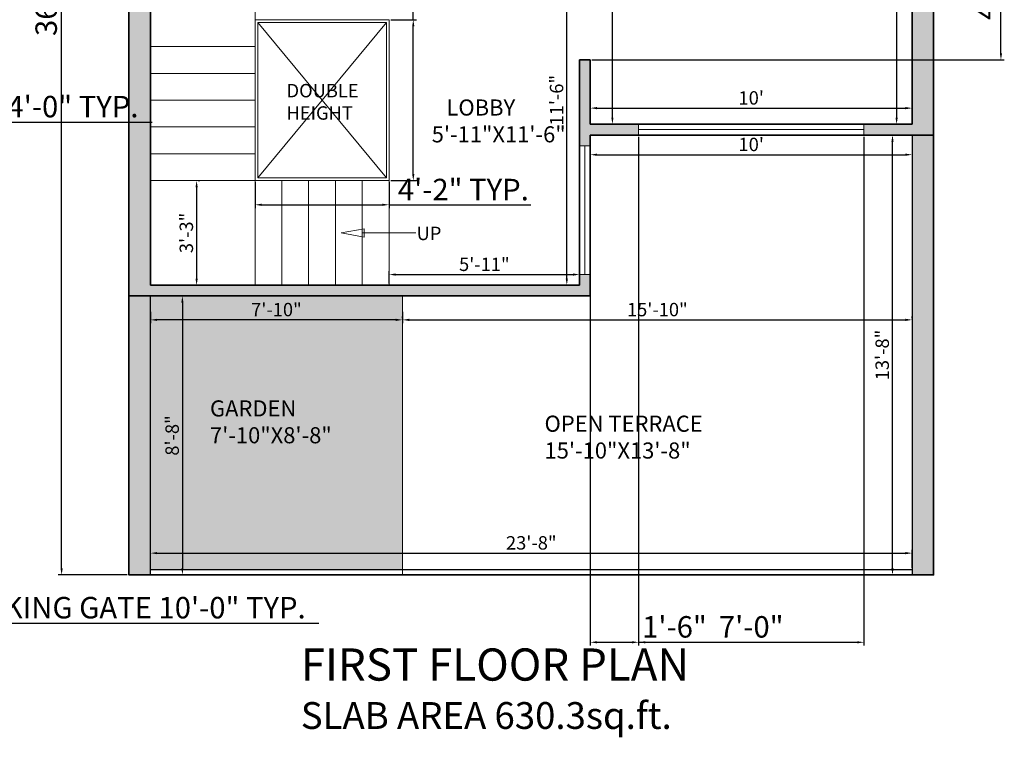
# Model space of a CAD drawing. Units: inches. Extents: x 3259 to 4981, y 1402 to 2026.
# Tile 10 of 11: x 4614 to 4981, y 1415 to 1682. Entities that reach past the tile are written whole.
import ezdxf

# ---------------------------------------------------------------- set-up
doc = ezdxf.new("R2010")
doc.units = ezdxf.units.IN
for name, color, linetype, lineweight in [('A-ANNO-DIMS', 2, 'Continuous', 13), ('A-ANNO-SYMB', 7, 'Continuous', 13), ('A-ANNO-TITL', 7, 'Continuous', 25), ('A-AREA-IDEN', 7, 'Continuous', 18), ('A-DOOR', 3, 'Continuous', 18), ('A-FLOR-STRS', 7, 'Continuous', 18), ('A-GLAZ', 4, 'Continuous', 18), ('A-WALL', 7, 'Continuous', 35), ('A-WALL-PATT', 252, 'Continuous', 13), ('A-WALL-PRPT', 7, 'Continuous', 25), ('L-PLNT', 3, 'Continuous', 18)]:
    doc.layers.add(name, color=color, linetype=linetype, lineweight=lineweight)
doc.layers.add('A-WALL-PRPT-PATT', color=9, linetype='Continuous', lineweight=13, true_color=0xc7c8ca)
doc.layers.add('L-PLNT-PATT', color=114, linetype='Continuous', lineweight=13, true_color=0x139b48)
doc.styles.get("Standard").update_dxf_attribs({"font": 'arial.ttf'})
doc.dimstyles.new('ISO-25', dxfattribs={"dimtxt": 8, "dimasz": 2.5, "dimexe": 1.25, "dimexo": 0.625, "dimtad": 1, "dimdec": 1, "dimlunit": 3, "dimtxsty": 'Standard', "dimcen": 2.5, "dimclrd": 4, "dimclre": 4, "dimclrt": 1, "dimadec": 0, "dimazin": 0, "dimtfac": 1, "dimtdec": 1, "dimtmove": 0, "dimatfit": 3, "dimfxl": 1, "dimarcsym": 0})

# ---------------------------------------------------------------- blocks, each defined once
blk = doc.blocks.new('*D90')
at = {"layer": 'A-ANNO-DIMS', "color": 0, "lineweight": -2, "transparency": 16777216}
for p, q in [((4662.83, 1573.27), (4662.83, 1568.97)), ((4756.83, 1573.27), (4756.83, 1568.97)), ((4754.33, 1570.22), (4665.33, 1570.22))]:
    blk.add_line(p, q, dxfattribs=at)
at = {"layer": 'A-ANNO-DIMS', "color": 0, "transparency": 16777216}
for points in [[(4665.33, 1570.63), (4665.33, 1569.8), (4662.83, 1570.22)], [(4754.33, 1570.63), (4754.33, 1569.8), (4756.83, 1570.22)]]:
    blk.add_solid(points, dxfattribs=at)
at = {"layer": 'Defpoints', "color": 0, "transparency": 16777216}
for p in [(4662.83, 1573.89), (4756.83, 1573.89), (4662.83, 1570.22)]:
    blk.add_point(p, dxfattribs=at)
at = {"layer": 'A-ANNO-DIMS', "color": 0, "transparency": 16777216, "insert": (4709.83, 1573.4), "char_height": 5, "attachment_point": 5}
blk.add_mtext('7\'-10"', dxfattribs=at)
blk = doc.blocks.new('*D91')
at = {"layer": 'A-ANNO-DIMS', "color": 0, "lineweight": -2, "transparency": 16777216}
for p, q in [((4673.41, 1579.12), (4676.02, 1579.12)), ((4674.77, 1576.62), (4674.77, 1477.62)), ((4673.41, 1475.12), (4676.02, 1475.12))]:
    blk.add_line(p, q, dxfattribs=at)
at = {"layer": 'A-ANNO-DIMS', "color": 0, "transparency": 16777216}
for points in [[(4674.35, 1576.62), (4675.18, 1576.62), (4674.77, 1579.12)], [(4674.35, 1477.62), (4675.18, 1477.62), (4674.77, 1475.12)]]:
    blk.add_solid(points, dxfattribs=at)
at = {"layer": 'Defpoints', "color": 0, "transparency": 16777216}
for p in [(4672.79, 1579.12), (4672.79, 1475.12), (4674.77, 1475.12)]:
    blk.add_point(p, dxfattribs=at)
at = {"layer": 'A-ANNO-DIMS', "color": 0, "transparency": 16777216, "insert": (4671.59, 1527.12), "char_height": 5, "attachment_point": 5, "rotation": 90}
blk.add_mtext('8\'-8"', dxfattribs=at)
blk = doc.blocks.new('*D92')
at = {"layer": 'A-ANNO-DIMS', "color": 0, "lineweight": -2, "transparency": 16777216}
for p, q in [((4756.83, 1570.84), (4756.83, 1571.47)), ((4946.83, 1570.84), (4946.83, 1571.47)), ((4759.33, 1570.22), (4944.33, 1570.22))]:
    blk.add_line(p, q, dxfattribs=at)
at = {"layer": 'A-ANNO-DIMS', "color": 0, "transparency": 16777216}
for points in [[(4759.33, 1570.63), (4759.33, 1569.8), (4756.83, 1570.22)], [(4944.33, 1570.63), (4944.33, 1569.8), (4946.83, 1570.22)]]:
    blk.add_solid(points, dxfattribs=at)
at = {"layer": 'Defpoints', "color": 0, "transparency": 16777216}
for p in [(4756.83, 1570.22), (4946.83, 1570.22), (4946.83, 1570.22)]:
    blk.add_point(p, dxfattribs=at)
at = {"layer": 'A-ANNO-DIMS', "color": 0, "transparency": 16777216, "insert": (4851.83, 1573.4), "char_height": 5, "attachment_point": 5}
blk.add_mtext('15\'-10"', dxfattribs=at)
blk = doc.blocks.new('*D93')
at = {"layer": 'A-ANNO-DIMS', "color": 0, "lineweight": -2, "transparency": 16777216}
for p, q in [((4946.2, 1639.12), (4938.24, 1639.12)), ((4939.49, 1477.62), (4939.49, 1636.62)), ((4946.2, 1475.12), (4938.24, 1475.12))]:
    blk.add_line(p, q, dxfattribs=at)
at = {"layer": 'A-ANNO-DIMS', "color": 0, "transparency": 16777216}
for points in [[(4939.08, 1636.62), (4939.91, 1636.62), (4939.49, 1639.12)], [(4939.08, 1477.62), (4939.91, 1477.62), (4939.49, 1475.12)]]:
    blk.add_solid(points, dxfattribs=at)
at = {"layer": 'Defpoints', "color": 0, "transparency": 16777216}
for p in [(4939.49, 1639.12), (4946.83, 1639.12), (4946.83, 1475.12)]:
    blk.add_point(p, dxfattribs=at)
at = {"layer": 'A-ANNO-DIMS', "color": 0, "transparency": 16777216, "insert": (4936.31, 1557.12), "char_height": 5, "attachment_point": 5, "rotation": 90}
blk.add_mtext('13\'-8"', dxfattribs=at)
blk = doc.blocks.new('*D85')
at = {"layer": 'A-ANNO-DIMS', "color": 0, "lineweight": -2, "transparency": 16777216}
for p, q in [((4751.83, 1583.74), (4751.83, 1588.35)), ((4754.33, 1587.1), (4820.33, 1587.1)), ((4822.83, 1583.74), (4822.83, 1588.35))]:
    blk.add_line(p, q, dxfattribs=at)
at = {"layer": 'A-ANNO-DIMS', "color": 0, "transparency": 16777216}
for points in [[(4754.33, 1587.52), (4754.33, 1586.68), (4751.83, 1587.1)], [(4820.33, 1587.52), (4820.33, 1586.68), (4822.83, 1587.1)]]:
    blk.add_solid(points, dxfattribs=at)
at = {"layer": 'Defpoints', "color": 0, "transparency": 16777216}
for p in [(4822.83, 1587.1), (4751.83, 1583.12), (4822.83, 1583.12)]:
    blk.add_point(p, dxfattribs=at)
at = {"layer": 'A-ANNO-DIMS', "color": 0, "transparency": 16777216, "insert": (4787.33, 1590.28), "char_height": 5, "attachment_point": 5}
blk.add_mtext('5\'-11"', dxfattribs=at)
blk = doc.blocks.new('*D86')
at = {"layer": 'A-ANNO-DIMS', "color": 0, "lineweight": -2, "transparency": 16777216}
for p, q in [((4787.45, 1721.12), (4819.32, 1721.12)), ((4818.07, 1585.62), (4818.07, 1718.62)), ((4822.2, 1583.12), (4816.82, 1583.12))]:
    blk.add_line(p, q, dxfattribs=at)
at = {"layer": 'A-ANNO-DIMS', "color": 0, "transparency": 16777216}
for points in [[(4817.66, 1718.62), (4818.49, 1718.62), (4818.07, 1721.12)], [(4817.66, 1585.62), (4818.49, 1585.62), (4818.07, 1583.12)]]:
    blk.add_solid(points, dxfattribs=at)
at = {"layer": 'Defpoints', "color": 0, "transparency": 16777216}
for p in [(4786.83, 1721.12), (4818.07, 1721.12), (4822.83, 1583.12)]:
    blk.add_point(p, dxfattribs=at)
at = {"layer": 'A-ANNO-DIMS', "color": 0, "transparency": 16777216, "insert": (4814.9, 1652.12), "char_height": 5, "attachment_point": 5, "rotation": 90}
blk.add_mtext('11\'-6"', dxfattribs=at)
blk = doc.blocks.new('*D87')
at = {"layer": 'A-ANNO-DIMS', "color": 0, "lineweight": -2, "transparency": 16777216}
for p, q in [((4826.83, 1643.74), (4826.83, 1650.4)), ((4829.33, 1649.15), (4944.33, 1649.15)), ((4946.83, 1643.74), (4946.83, 1650.4))]:
    blk.add_line(p, q, dxfattribs=at)
at = {"layer": 'A-ANNO-DIMS', "color": 0, "transparency": 16777216}
for points in [[(4829.33, 1649.56), (4829.33, 1648.73), (4826.83, 1649.15)], [(4944.33, 1649.56), (4944.33, 1648.73), (4946.83, 1649.15)]]:
    blk.add_solid(points, dxfattribs=at)
at = {"layer": 'Defpoints', "color": 0, "transparency": 16777216}
for p in [(4946.83, 1649.15), (4826.83, 1643.12), (4946.83, 1643.12)]:
    blk.add_point(p, dxfattribs=at)
at = {"layer": 'A-ANNO-DIMS', "color": 0, "transparency": 16777216, "insert": (4886.83, 1652.32), "char_height": 5, "attachment_point": 5}
blk.add_mtext("10'", dxfattribs=at)
blk = doc.blocks.new('*D88')
at = {"layer": 'A-ANNO-DIMS', "color": 0, "lineweight": -2, "transparency": 16777216}
for p, q in [((4827.45, 1847.12), (4836.33, 1847.12)), ((4835.08, 1645.62), (4835.08, 1844.62)), ((4827.45, 1643.12), (4836.33, 1643.12))]:
    blk.add_line(p, q, dxfattribs=at)
at = {"layer": 'A-ANNO-DIMS', "color": 0, "transparency": 16777216}
for points in [[(4834.66, 1844.62), (4835.49, 1844.62), (4835.08, 1847.12)], [(4834.66, 1645.62), (4835.49, 1645.62), (4835.08, 1643.12)]]:
    blk.add_solid(points, dxfattribs=at)
at = {"layer": 'Defpoints', "color": 0, "transparency": 16777216}
for p in [(4826.83, 1847.12), (4835.08, 1847.12), (4826.83, 1643.12)]:
    blk.add_point(p, dxfattribs=at)
at = {"layer": 'A-ANNO-DIMS', "color": 0, "transparency": 16777216, "insert": (4831.94, 1745.12), "char_height": 5, "attachment_point": 5, "rotation": 90}
blk.add_mtext("17'", dxfattribs=at)
blk = doc.blocks.new('*D94')
at = {"layer": 'A-ANNO-DIMS', "color": 0, "lineweight": -2, "transparency": 16777216}
for p, q in [((4680.06, 1619.62), (4680.06, 1585.62)), ((4680.69, 1622.12), (4681.31, 1622.12)), ((4680.69, 1583.12), (4681.31, 1583.12))]:
    blk.add_line(p, q, dxfattribs=at)
at = {"layer": 'A-ANNO-DIMS', "color": 0, "transparency": 16777216}
for points in [[(4679.64, 1619.62), (4680.48, 1619.62), (4680.06, 1622.12)], [(4679.64, 1585.62), (4680.48, 1585.62), (4680.06, 1583.12)]]:
    blk.add_solid(points, dxfattribs=at)
at = {"layer": 'Defpoints', "color": 0, "transparency": 16777216}
for p in [(4680.06, 1622.12), (4680.06, 1583.12), (4680.06, 1583.12)]:
    blk.add_point(p, dxfattribs=at)
at = {"layer": 'A-ANNO-DIMS', "color": 0, "transparency": 16777216, "insert": (4676.88, 1602.62), "char_height": 5, "attachment_point": 5, "rotation": 90}
blk.add_mtext('3\'-3"', dxfattribs=at)
blk = doc.blocks.new('*D63')
at = {"layer": 'A-ANNO-DIMS', "color": 0, "lineweight": -2, "transparency": 16777216}
for p, q in [((4826.83, 1638.49), (4826.83, 1630.53)), ((4946.83, 1638.49), (4946.83, 1630.53)), ((4829.33, 1631.78), (4944.33, 1631.78))]:
    blk.add_line(p, q, dxfattribs=at)
at = {"layer": 'A-ANNO-DIMS', "color": 0, "transparency": 16777216}
for points in [[(4829.33, 1632.2), (4829.33, 1631.37), (4826.83, 1631.78)], [(4944.33, 1632.2), (4944.33, 1631.37), (4946.83, 1631.78)]]:
    blk.add_solid(points, dxfattribs=at)
at = {"layer": 'Defpoints', "color": 0, "transparency": 16777216}
for p in [(4826.83, 1639.12), (4946.83, 1639.12), (4946.83, 1631.78)]:
    blk.add_point(p, dxfattribs=at)
at = {"layer": 'A-ANNO-DIMS', "color": 0, "transparency": 16777216, "insert": (4886.83, 1634.96), "char_height": 5, "attachment_point": 5}
blk.add_mtext("10'", dxfattribs=at)
blk = doc.blocks.new('*D99')
at = {"layer": 'A-ANNO-DIMS', "color": 0, "lineweight": -2, "transparency": 16777216}
for p, q in [((4946.2, 1847.12), (4939.77, 1847.12)), ((4941.02, 1844.62), (4941.02, 1645.62)), ((4946.2, 1643.12), (4939.77, 1643.12))]:
    blk.add_line(p, q, dxfattribs=at)
at = {"layer": 'A-ANNO-DIMS', "color": 0, "transparency": 16777216}
for points in [[(4940.61, 1844.62), (4941.44, 1844.62), (4941.02, 1847.12)], [(4940.61, 1645.62), (4941.44, 1645.62), (4941.02, 1643.12)]]:
    blk.add_solid(points, dxfattribs=at)
at = {"layer": 'Defpoints', "color": 0, "transparency": 16777216}
for p in [(4946.83, 1847.12), (4941.02, 1643.12), (4946.83, 1643.12)]:
    blk.add_point(p, dxfattribs=at)
at = {"layer": 'A-ANNO-DIMS', "color": 0, "transparency": 16777216, "insert": (4937.89, 1745.12), "char_height": 5, "attachment_point": 5, "rotation": 90}
blk.add_mtext("17'", dxfattribs=at)
blk = doc.blocks.new('*D133')
at = {"layer": 'A-ANNO-DIMS', "color": 0, "lineweight": -2, "transparency": 16777216}
for p, q in [((4662.83, 1477.74), (4662.83, 1484.5)), ((4665.33, 1483.25), (4944.33, 1483.25)), ((4946.83, 1477.74), (4946.83, 1484.5))]:
    blk.add_line(p, q, dxfattribs=at)
at = {"layer": 'A-ANNO-DIMS', "color": 0, "transparency": 16777216}
for points in [[(4665.33, 1483.67), (4665.33, 1482.84), (4662.83, 1483.25)], [(4944.33, 1483.67), (4944.33, 1482.84), (4946.83, 1483.25)]]:
    blk.add_solid(points, dxfattribs=at)
at = {"layer": 'Defpoints', "color": 0, "transparency": 16777216}
for p in [(4946.83, 1483.25), (4662.83, 1477.12), (4946.83, 1477.12)]:
    blk.add_point(p, dxfattribs=at)
at = {"layer": 'A-ANNO-DIMS', "color": 0, "transparency": 16777216, "insert": (4804.83, 1486.43), "char_height": 5, "attachment_point": 5}
blk.add_mtext('23\'-8"', dxfattribs=at)
blk = doc.blocks.new('STAIR-WELL-50x60')
for p, q in [((1, 59), (49, 1)), ((1, 1), (49, 59))]:
    blk.add_line(p, q)
for points in [[(50, 60), (0, 60), (0, 0), (50, 0)], [(49, 59), (1, 59), (1, 1), (49, 1)]]:
    blk.add_lwpolyline(points, close=True)
blk = doc.blocks.new('STAIR-DIRECTION')
blk.add_line((7.93, 1.55), (27.85, 1.55))
blk.add_lwpolyline([(0, 1.55), (8.64, 3.11), (8.64, 0)], close=True)
blk = doc.blocks.new('*D154')
at = {"layer": 'A-ANNO-DIMS', "color": 4, "lineweight": -2, "transparency": 16777216}
for p, q in [((4760.83, 1682.12), (4760.83, 1804.15)), ((4752.45, 1682.12), (4762.08, 1682.12)), ((4760.83, 1624.62), (4760.83, 1679.62)), ((4752.45, 1622.12), (4762.08, 1622.12))]:
    blk.add_line(p, q, dxfattribs=at)
at = {"layer": 'A-ANNO-DIMS', "color": 4, "transparency": 16777216}
for points in [[(4760.41, 1679.62), (4761.25, 1679.62), (4760.83, 1682.12)], [(4760.41, 1624.62), (4761.25, 1624.62), (4760.83, 1622.12)]]:
    blk.add_solid(points, dxfattribs=at)
at = {"layer": 'Defpoints', "color": 0, "transparency": 16777216}
for p in [(4751.83, 1682.12), (4760.83, 1682.12), (4751.83, 1622.12)]:
    blk.add_point(p, dxfattribs=at)
at = {"layer": 'A-ANNO-DIMS', "color": 1, "transparency": 16777216, "insert": (4756.07, 1744.38), "char_height": 8, "attachment_point": 5, "rotation": 90}
blk.add_mtext('STAIR WELL 5\'-0" TYP.', dxfattribs=at)
blk = doc.blocks.new('*D155')
at = {"layer": 'A-ANNO-DIMS', "color": 4, "lineweight": -2, "transparency": 16777216}
for p, q in [((4701.83, 1621.49), (4701.83, 1611.87)), ((4751.83, 1621.49), (4751.83, 1611.87)), ((4704.33, 1613.12), (4749.33, 1613.12)), ((4751.83, 1613.12), (4804.67, 1613.12))]:
    blk.add_line(p, q, dxfattribs=at)
at = {"layer": 'A-ANNO-DIMS', "color": 4, "transparency": 16777216}
for points in [[(4704.33, 1613.53), (4704.33, 1612.7), (4701.83, 1613.12)], [(4749.33, 1613.53), (4749.33, 1612.7), (4751.83, 1613.12)]]:
    blk.add_solid(points, dxfattribs=at)
at = {"layer": 'Defpoints', "color": 0, "transparency": 16777216}
for p in [(4701.83, 1622.12), (4751.83, 1622.12), (4751.83, 1613.12)]:
    blk.add_point(p, dxfattribs=at)
at = {"layer": 'A-ANNO-DIMS', "color": 1, "transparency": 16777216, "insert": (4779.5, 1617.76), "char_height": 8, "attachment_point": 5}
blk.add_mtext('4\'-2" TYP.', dxfattribs=at)
blk = doc.blocks.new('*D170')
at = {"layer": 'A-ANNO-DIMS', "color": 4, "lineweight": -2, "transparency": 16777216}
for p, q in [((4478.33, 1650.49), (4478.33, 1642.67)), ((4526.33, 1650.49), (4526.33, 1642.67)), ((4480.83, 1643.92), (4523.83, 1643.92)), ((4526.33, 1643.92), (4663.49, 1643.92))]:
    blk.add_line(p, q, dxfattribs=at)
at = {"layer": 'A-ANNO-DIMS', "color": 4, "transparency": 16777216}
for points in [[(4480.83, 1644.33), (4480.83, 1643.5), (4478.33, 1643.92)], [(4523.83, 1644.33), (4523.83, 1643.5), (4526.33, 1643.92)]]:
    blk.add_solid(points, dxfattribs=at)
at = {"layer": 'Defpoints', "color": 0, "transparency": 16777216}
for p in [(4478.33, 1651.12), (4526.33, 1651.12), (4526.33, 1643.92)]:
    blk.add_point(p, dxfattribs=at)
at = {"layer": 'A-ANNO-DIMS', "color": 1, "transparency": 16777216, "insert": (4596.16, 1648.68), "char_height": 8, "attachment_point": 5}
blk.add_mtext('ENTRY DOORS 4\'-0" TYP.', dxfattribs=at)
blk = doc.blocks.new('*D172')
at = {"layer": 'A-ANNO-DIMS', "color": 4, "lineweight": -2, "transparency": 16777216}
for p, q in [((4460.33, 1474.49), (4460.33, 1455.87)), ((4580.33, 1474.49), (4580.33, 1455.87)), ((4462.83, 1457.12), (4577.83, 1457.12)), ((4580.33, 1457.12), (4725.6, 1457.12))]:
    blk.add_line(p, q, dxfattribs=at)
at = {"layer": 'A-ANNO-DIMS', "color": 4, "transparency": 16777216}
for points in [[(4462.83, 1457.53), (4462.83, 1456.7), (4460.33, 1457.12)], [(4577.83, 1457.53), (4577.83, 1456.7), (4580.33, 1457.12)]]:
    blk.add_solid(points, dxfattribs=at)
at = {"layer": 'Defpoints', "color": 0, "transparency": 16777216}
for p in [(4460.33, 1475.12), (4580.33, 1475.12), (4580.33, 1457.12)]:
    blk.add_point(p, dxfattribs=at)
at = {"layer": 'A-ANNO-DIMS', "color": 1, "transparency": 16777216, "insert": (4654.22, 1461.88), "char_height": 8, "attachment_point": 5}
blk.add_mtext('PARKING GATE 10\'-0" TYP.', dxfattribs=at)
blk = doc.blocks.new('*D189')
at = {"layer": 'A-ANNO-DIMS', "color": 4, "lineweight": -2, "transparency": 16777216}
for p, q in [((4654.2, 1907.12), (4628.48, 1907.12)), ((4629.73, 1477.62), (4629.73, 1904.62)), ((4654.2, 1475.12), (4628.48, 1475.12))]:
    blk.add_line(p, q, dxfattribs=at)
at = {"layer": 'A-ANNO-DIMS', "color": 4, "transparency": 16777216}
for points in [[(4629.31, 1904.62), (4630.15, 1904.62), (4629.73, 1907.12)], [(4629.31, 1477.62), (4630.15, 1477.62), (4629.73, 1475.12)]]:
    blk.add_solid(points, dxfattribs=at)
at = {"layer": 'Defpoints', "color": 0, "transparency": 16777216}
for p in [(4629.73, 1907.12), (4654.83, 1907.12), (4654.83, 1475.12)]:
    blk.add_point(p, dxfattribs=at)
at = {"layer": 'A-ANNO-DIMS', "color": 1, "transparency": 16777216, "insert": (4625.02, 1691.12), "char_height": 8, "attachment_point": 5, "rotation": 90}
blk.add_mtext('36\'-0"', dxfattribs=at)
blk = doc.blocks.new('*D197')
at = {"layer": 'A-ANNO-DIMS', "color": 4, "lineweight": -2, "transparency": 16777216}
for p, q in [((4827.45, 1721.12), (4981.18, 1721.12)), ((4979.93, 1669.62), (4979.93, 1718.62)), ((4827.45, 1667.12), (4981.18, 1667.12))]:
    blk.add_line(p, q, dxfattribs=at)
at = {"layer": 'A-ANNO-DIMS', "color": 4, "transparency": 16777216}
for points in [[(4979.51, 1718.62), (4980.35, 1718.62), (4979.93, 1721.12)], [(4979.51, 1669.62), (4980.35, 1669.62), (4979.93, 1667.12)]]:
    blk.add_solid(points, dxfattribs=at)
at = {"layer": 'Defpoints', "color": 0, "transparency": 16777216}
for p in [(4826.83, 1721.12), (4979.93, 1721.12), (4826.83, 1667.12)]:
    blk.add_point(p, dxfattribs=at)
at = {"layer": 'A-ANNO-DIMS', "color": 1, "transparency": 16777216, "insert": (4975.22, 1694.12), "char_height": 8, "attachment_point": 5, "rotation": 90}
blk.add_mtext('4\'-6"', dxfattribs=at)
blk = doc.blocks.new('*D198')
at = {"layer": 'A-ANNO-DIMS', "color": 4, "lineweight": -2, "transparency": 16777216}
for p, q in [((4844.83, 1638.49), (4844.83, 1448.77)), ((4928.83, 1638.49), (4928.83, 1448.77)), ((4847.33, 1450.02), (4926.33, 1450.02))]:
    blk.add_line(p, q, dxfattribs=at)
at = {"layer": 'A-ANNO-DIMS', "color": 4, "transparency": 16777216}
for points in [[(4847.33, 1450.43), (4847.33, 1449.6), (4844.83, 1450.02)], [(4926.33, 1450.43), (4926.33, 1449.6), (4928.83, 1450.02)]]:
    blk.add_solid(points, dxfattribs=at)
at = {"layer": 'Defpoints', "color": 0, "transparency": 16777216}
for p in [(4844.83, 1639.12), (4928.83, 1639.12), (4928.83, 1450.02)]:
    blk.add_point(p, dxfattribs=at)
at = {"layer": 'A-ANNO-DIMS', "color": 1, "transparency": 16777216, "insert": (4886.83, 1454.73), "char_height": 8, "attachment_point": 5}
blk.add_mtext('7\'-0"', dxfattribs=at)
blk = doc.blocks.new('*D199')
at = {"layer": 'A-ANNO-DIMS', "color": 4, "lineweight": -2, "transparency": 16777216}
for p, q in [((4826.83, 1638.49), (4826.83, 1448.77)), ((4844.83, 1638.49), (4844.83, 1448.77)), ((4829.33, 1450.02), (4842.33, 1450.02)), ((4844.83, 1450.02), (4869.09, 1450.02))]:
    blk.add_line(p, q, dxfattribs=at)
at = {"layer": 'A-ANNO-DIMS', "color": 4, "transparency": 16777216}
for points in [[(4829.33, 1450.43), (4829.33, 1449.6), (4826.83, 1450.02)], [(4842.33, 1450.43), (4842.33, 1449.6), (4844.83, 1450.02)]]:
    blk.add_solid(points, dxfattribs=at)
at = {"layer": 'Defpoints', "color": 0, "transparency": 16777216}
for p in [(4826.83, 1639.12), (4844.83, 1639.12), (4844.83, 1450.02)]:
    blk.add_point(p, dxfattribs=at)
at = {"layer": 'A-ANNO-DIMS', "color": 1, "transparency": 16777216, "insert": (4858.21, 1454.73), "char_height": 8, "attachment_point": 5}
blk.add_mtext('1\'-6"', dxfattribs=at)

msp = doc.modelspace()

# ---------------------------------------------------------------- hatches: boundary and pattern name
at = {"layer": 'A-WALL-PATT'}
h = msp.add_hatch(color=256, dxfattribs=at)
h.dxf.hatch_style = 1
h.paths.add_polyline_path([(4826.83, 1851.12), (4822.83, 1851.12), (4822.83, 1721.12), (4826.83, 1721.12), (4826.83, 1777.43), (4826.82, 1777.43), (4826.82, 1777.47), (4826.83, 1777.47), (4826.83, 1781.5), (4826.83, 1781.5), (4826.83, 1781.55)], flags=17)
h.paths.add_polyline_path([(4786.83, 1863.12), (4782.83, 1863.12), (4782.83, 1851.12), (4698.83, 1851.12), (4698.83, 1847.12), (4736.66, 1847.12), (4736.66, 1847.13), (4736.7, 1847.13), (4736.7, 1847.12), (4740.73, 1847.12), (4740.73, 1847.12), (4740.78, 1847.12), (4786.83, 1847.12)], flags=17)
h.paths.add_polyline_path([(4862.83, 1863.12), (4858.83, 1863.12), (4858.83, 1847.12), (4862.83, 1847.12)], flags=17)
h.paths.add_polyline_path([(4954.83, 1907.12), (4654.83, 1907.12), (4654.83, 1579.12), (4826.83, 1579.12), (4826.83, 1587.12), (4822.83, 1587.12), (4822.83, 1583.12), (4662.83, 1583.12), (4662.83, 1721.12), (4786.83, 1721.12), (4786.83, 1725.12), (4662.83, 1725.12), (4662.83, 1899.12), (4698.83, 1899.12), (4698.83, 1881.12), (4702.83, 1881.12), (4702.83, 1899.12), (4782.83, 1899.12), (4782.83, 1887.12), (4786.83, 1887.12), (4786.83, 1899.12), (4858.83, 1899.12), (4858.83, 1887.12), (4862.83, 1887.12), (4862.83, 1899.12), (4946.83, 1899.12), (4946.83, 1851.12), (4892.83, 1851.12), (4892.83, 1847.12), (4946.83, 1847.12), (4946.83, 1643.12), (4928.83, 1643.12), (4928.83, 1639.12), (4954.83, 1639.12)])
h.paths.add_polyline_path([(4826.83, 1667.12), (4822.83, 1667.12), (4822.83, 1635.12), (4826.83, 1635.12), (4826.83, 1639.12), (4844.83, 1639.12), (4844.83, 1643.12), (4826.83, 1643.12)], flags=17)
at = {"layer": 'A-WALL-PRPT-PATT'}
h = msp.add_hatch(color=256, dxfattribs=at)
h.dxf.hatch_style = 1
h.paths.add_polyline_path([(4954.83, 1639.12), (4946.83, 1639.12), (4946.83, 1475.12), (4954.83, 1475.12)])
h.paths.add_polyline_path([(4662.83, 1579.12), (4654.83, 1579.12), (4654.83, 1475.12), (4662.83, 1475.12)])
at = {"layer": 'L-PLNT-PATT'}
h = msp.add_hatch(color=256, dxfattribs=at)
h.dxf.hatch_style = 1
h.paths.add_polyline_path([(4756.83, 1579.12), (4662.83, 1579.12), (4662.83, 1477.12), (4756.83, 1477.12)])
h.paths.add_polyline_path([(4683.1, 1520.8), (4729.79, 1520.8), (4729.79, 1543.19), (4683.1, 1543.19)], flags=24)

# ---------------------------------------------------------------- linework, layer by layer
at = {"layer": 'A-DOOR'}
for p, q in [((4822.83, 1635.12), (4826.83, 1635.12)), ((4824.83, 1635.12), (4824.83, 1587.12)), ((4826.83, 1587.12), (4822.83, 1587.12))]:
    msp.add_line(p, q, dxfattribs=at)
at = {"layer": 'A-FLOR-STRS'}
for p, q in [((4701.83, 1583.12), (4701.83, 1721.12)), ((4662.83, 1672.12), (4701.83, 1672.12)), ((4662.83, 1662.12), (4701.83, 1662.12)), ((4662.83, 1652.12), (4701.83, 1652.12)), ((4662.83, 1642.12), (4701.83, 1642.12)), ((4662.83, 1632.12), (4701.83, 1632.12)), ((4751.83, 1622.12), (4662.83, 1622.12)), ((4711.83, 1583.12), (4711.83, 1622.12)), ((4721.83, 1583.12), (4721.83, 1622.12)), ((4731.83, 1583.12), (4731.83, 1622.12)), ((4741.83, 1583.12), (4741.83, 1622.12)), ((4751.83, 1583.12), (4751.83, 1622.12))]:
    msp.add_line(p, q, dxfattribs=at)
at = {"layer": 'A-GLAZ'}
for p, q in [((4844.83, 1639.12), (4844.83, 1643.12)), ((4844.83, 1641.12), (4928.83, 1641.12)), ((4928.83, 1639.12), (4928.83, 1643.12))]:
    msp.add_line(p, q, dxfattribs=at)
at = {"layer": 'A-WALL'}
for p, q in [((4946.83, 1847.12), (4946.83, 1643.12)), ((4662.83, 1583.12), (4662.83, 1721.12)), ((4822.83, 1583.12), (4822.83, 1667.12)), ((4822.83, 1667.12), (4826.83, 1667.12)), ((4826.83, 1643.12), (4826.83, 1667.12)), ((4826.83, 1643.12), (4946.83, 1643.12)), ((4826.83, 1639.12), (4954.83, 1639.12)), ((4826.83, 1579.12), (4826.83, 1639.12)), ((4822.83, 1583.12), (4662.83, 1583.12)), ((4826.83, 1579.12), (4654.83, 1579.12))]:
    msp.add_line(p, q, dxfattribs=at)
msp.add_lwpolyline([(4946.83, 1475.12), (4654.83, 1475.12), (4654.83, 1907.12), (4954.83, 1907.12), (4954.83, 1475.12), (4946.83, 1475.12)], dxfattribs=at)
at = {"layer": 'A-WALL-PRPT'}
for p, q in [((4946.83, 1639.12), (4946.83, 1475.12)), ((4662.83, 1475.12), (4662.83, 1579.12)), ((4662.83, 1477.12), (4946.83, 1477.12))]:
    msp.add_line(p, q, dxfattribs=at)
at = {"layer": 'L-PLNT'}
msp.add_line((4756.83, 1475.12), (4756.83, 1579.12), dxfattribs=at)

# ---------------------------------------------------------------- block references
at = {"layer": 'A-ANNO-SYMB'}
msp.add_blockref('STAIR-DIRECTION', (4733.94, 1601.06), dxfattribs=at)
at = {"layer": 'A-FLOR-STRS'}
msp.add_blockref('STAIR-WELL-50x60', (4701.83, 1622.12), dxfattribs=at)

# ---------------------------------------------------------------- texts
at = {"layer": 'A-ANNO-SYMB', "insert": (4771.31, 1604.94), "char_height": 5, "attachment_point": 3}
msp.add_mtext_dynamic_manual_height_columns('UP', width=10.7355, gutter_width=12.5, heights=[0], dxfattribs=at)
at = {"layer": 'A-ANNO-TITL', "insert": (4718.91, 1447.72), "char_height": 12, "attachment_point": 1}
msp.add_mtext_dynamic_manual_height_columns('FIRST FLOOR PLAN\\P{\\H0.83333x;SLAB AREA 630.3sq.ft.}', width=298.7081, gutter_width=12.5, heights=[0], dxfattribs=at)
at = {"layer": 'A-AREA-IDEN', "attachment_point": 1}
for s, insert, char_height in [('DOUBLE\\PHEIGHT', (4713.59, 1658.17), 5), ('   LOBBY\\P5\'-11"X11\'-6"', (4767.71, 1652.38), 6), ('GARDEN\\P7\'-10"X8\'-8"', (4685.05, 1540.2), 6), ('OPEN TERRACE\\P15\'-10"X13\'-8"', (4809.77, 1534.51), 6)]:
    msp.add_mtext_dynamic_manual_height_columns(s, width=127.3061, gutter_width=12.5, heights=[0], dxfattribs=dict(at, insert=insert, char_height=char_height))

# ---------------------------------------------------------------- dimensions: what is measured, and where the dimension line sits
at = {"layer": 'A-ANNO-DIMS'}
for base, p1, p2, override, picture, middle in [((4629.73, 1907.12), (4654.83, 1475.12), (4654.83, 1907.12), {"dimdec": 1, "dimlfac": 1, "dimrnd": 0, "dimzin": 1, "dimdsep": 46, "dimlunit": 4, "dimfrac": 2}, '*D189', (4625.02, 1691.12)), ((4835.08, 1847.12), (4826.83, 1643.12), (4826.83, 1847.12), {"dimtxt": 5, "dimclrd": 0, "dimclre": 0, "dimclrt": 0}, '*D88', (4831.94, 1745.12)), ((4941.02, 1643.12), (4946.83, 1847.12), (4946.83, 1643.12), {"dimtxt": 5, "dimclrd": 0, "dimclre": 0, "dimclrt": 0}, '*D99', (4937.89, 1745.12)), ((4818.07, 1721.12), (4822.83, 1583.12), (4786.83, 1721.12), {"dimtxt": 5, "dimclrd": 0, "dimclre": 0, "dimclrt": 0}, '*D86', (4814.9, 1652.12)), ((4979.93, 1721.12), (4826.83, 1667.12), (4826.83, 1721.12), {"dimdec": 1, "dimlfac": 1, "dimrnd": 0, "dimzin": 1, "dimdsep": 46, "dimlunit": 4, "dimfrac": 2}, '*D197', (4975.22, 1694.12)), ((4939.49, 1639.12), (4946.83, 1475.12), (4946.83, 1639.12), {"dimtxt": 5, "dimclrd": 0, "dimclre": 0, "dimclrt": 0}, '*D93', (4936.31, 1557.12)), ((4680.06, 1583.12), (4680.06, 1622.12), (4680.06, 1583.12), {"dimtxt": 5, "dimclrd": 0, "dimclre": 0, "dimclrt": 0}, '*D94', (4676.88, 1602.62)), ((4674.77, 1475.12), (4672.79, 1579.12), (4672.79, 1475.12), {"dimtxt": 5, "dimclrd": 0, "dimclre": 0, "dimclrt": 0}, '*D91', (4671.59, 1527.12))]:
    dim = msp.add_linear_dim(base=base, p1=p1, p2=p2, angle=90, dimstyle='ISO-25', override=override, dxfattribs=at)
    dim.commit()
    dim.dimension.update_dxf_attribs({"geometry": picture, "text_midpoint": middle})
dim = msp.add_linear_dim(base=(4760.83, 1682.12), p1=(4751.83, 1622.12), p2=(4751.83, 1682.12), angle=90, text='STAIR WELL <> TYP.', dimstyle='ISO-25', override={"dimdec": 1, "dimlfac": 1, "dimrnd": 0, "dimzin": 1, "dimdsep": 46, "dimlunit": 4, "dimfrac": 2}, dxfattribs=at)
dim.commit()
dim.dimension.update_dxf_attribs({"geometry": '*D154', "text_midpoint": (4756.07, 1744.38)})
for base, p1, p2, text, picture, middle in [((4526.33, 1643.92), (4478.33, 1651.12), (4526.33, 1651.12), 'ENTRY DOORS <> TYP.', '*D170', (4596.16, 1648.68)), ((4751.83, 1613.12), (4701.83, 1622.12), (4751.83, 1622.12), '<> TYP.', '*D155', (4779.5, 1617.76)), ((4580.33, 1457.12), (4460.33, 1475.12), (4580.33, 1475.12), 'PARKING GATE <> TYP.', '*D172', (4654.22, 1461.88))]:
    dim = msp.add_linear_dim(base=base, p1=p1, p2=p2, text=text, dimstyle='ISO-25', override={"dimdec": 1, "dimlfac": 1, "dimrnd": 0, "dimzin": 1, "dimdsep": 46, "dimlunit": 4, "dimfrac": 2}, dxfattribs=at)
    dim.commit()
    dim.dimension.update_dxf_attribs({"geometry": picture, "text_midpoint": middle})
for base, p1, p2, override, picture, middle in [((4946.83, 1649.15), (4826.83, 1643.12), (4946.83, 1643.12), {"dimtxt": 5, "dimclrd": 0, "dimclre": 0, "dimclrt": 0}, '*D87', (4886.83, 1652.32)), ((4946.83, 1631.78), (4826.83, 1639.12), (4946.83, 1639.12), {"dimtxt": 5, "dimclrd": 0, "dimclre": 0, "dimclrt": 0}, '*D63', (4886.83, 1634.96)), ((4844.83, 1450.02), (4826.83, 1639.12), (4844.83, 1639.12), {"dimdec": 1, "dimlfac": 1, "dimrnd": 0, "dimzin": 1, "dimdsep": 46, "dimlunit": 4, "dimfrac": 2}, '*D199', (4858.21, 1454.73)), ((4928.83, 1450.02), (4844.83, 1639.12), (4928.83, 1639.12), {"dimdec": 1, "dimlfac": 1, "dimrnd": 0, "dimzin": 1, "dimdsep": 46, "dimlunit": 4, "dimfrac": 2}, '*D198', (4886.83, 1454.73)), ((4822.83, 1587.1), (4751.83, 1583.12), (4822.83, 1583.12), {"dimtxt": 5, "dimclrd": 0, "dimclre": 0, "dimclrt": 0}, '*D85', (4787.33, 1590.28)), ((4662.83, 1570.22), (4756.83, 1573.89), (4662.83, 1573.89), {"dimtxt": 5, "dimclrd": 0, "dimclre": 0, "dimclrt": 0}, '*D90', (4709.83, 1573.4)), ((4946.83, 1570.22), (4756.83, 1570.22), (4946.83, 1570.22), {"dimtxt": 5, "dimclrd": 0, "dimclre": 0, "dimclrt": 0}, '*D92', (4851.83, 1573.4)), ((4946.83, 1483.25), (4662.83, 1477.12), (4946.83, 1477.12), {"dimtxt": 5, "dimclrd": 0, "dimclre": 0, "dimclrt": 0}, '*D133', (4804.83, 1486.43))]:
    dim = msp.add_linear_dim(base=base, p1=p1, p2=p2, dimstyle='ISO-25', override=override, dxfattribs=at)
    dim.commit()
    dim.dimension.update_dxf_attribs({"geometry": picture, "text_midpoint": middle})

doc.saveas('drawing.dxf')
